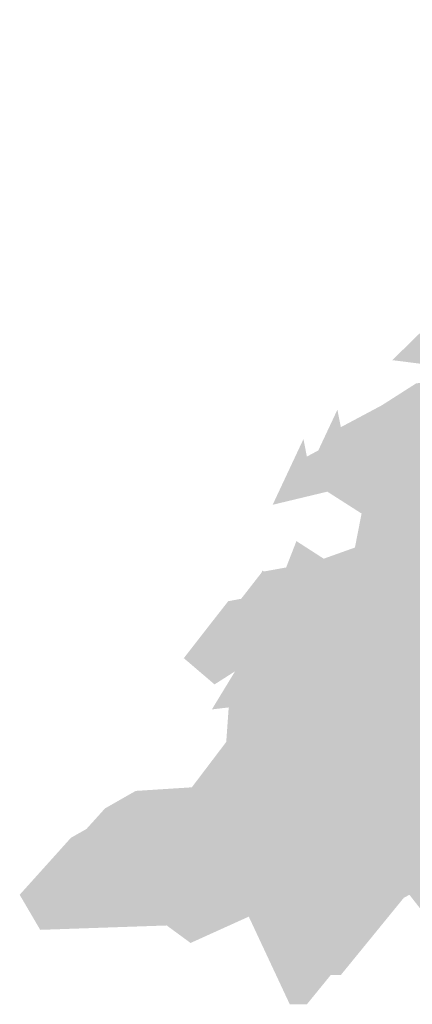
# Model space of a CAD drawing. Units: feet. Extents: x 2368 to 3224, y 836 to 1229.
# Tile 1 of 9: x 2390.53 to 2394.66, y 849.57 to 859.93. Entities that reach past the tile are written whole.
import ezdxf

# ---------------------------------------------------------------- set-up
doc = ezdxf.new("R2010")
doc.units = ezdxf.units.FT
doc.layers.add('L-PLNT', color=3, linetype='Continuous', lineweight=13)

msp = doc.modelspace()

# ---------------------------------------------------------------- hatches: boundary and pattern name
at = {"layer": 'L-PLNT'}
h = msp.add_hatch(color=256, dxfattribs=at)
h.dxf.hatch_style = 1
h.paths.add_polyline_path([(2401.097, 854.492), (2400.522, 855.091), (2399.803, 855.321), (2400.126, 855.828), (2399.839, 856.704), (2399.659, 856.704), (2399.3, 857.487), (2399.084, 857.441), (2398.832, 857.441), (2398.653, 857.809), (2398.76, 858.316), (2399.048, 858.316), (2398.509, 858.962), (2398.436, 859.473), (2398.149, 859.791), (2397.898, 859.514), (2397.754, 859.607), (2397.718, 859.837), (2397.538, 859.929), (2397.287, 859.699), (2396.999, 859.745), (2396.783, 859.33), (2396.783, 858.962), (2397.071, 858.823), (2396.855, 858.685), (2396.64, 858.869), (2396.029, 858.27), (2396.029, 858.132), (2395.777, 857.994), (2395.849, 857.856), (2396.029, 857.579), (2395.705, 857.349), (2395.382, 857.579), (2395.202, 857.533), (2395.13, 857.349), (2395.382, 857.303), (2395.418, 856.934), (2395.136, 856.98), (2394.806, 856.657), (2395.166, 856.611), (2395.022, 856.151), (2394.699, 856.104), (2394.339, 855.874), (2393.908, 855.644), (2393.872, 855.828), (2393.548, 855.137), (2394.124, 855.275), (2394.483, 855.045), (2394.375, 854.492), (2393.728, 854.261), (2393.441, 854.446), (2393.333, 854.169), (2393.081, 854.123), (2392.865, 853.846), (2392.614, 853.524), (2392.937, 853.247), (2393.153, 853.386), (2392.909, 852.985), (2393.086, 853.006), (2393.061, 852.643), (2392.47, 851.865), (2391.751, 851.819), (2391.428, 851.635), (2390.888, 851.035), (2391.104, 850.667), (2392.434, 850.713), (2392.686, 850.529), (2393.297, 850.805), (2393.728, 849.883), (2393.908, 849.883), (2394.735, 850.897), (2394.986, 851.035), (2395.166, 850.805), (2395.166, 850.483), (2395.453, 850.39), (2395.849, 850.39), (2395.993, 850.713), (2396.46, 850.943), (2396.927, 850.989), (2397.143, 851.174), (2397.179, 851.22), (2397.287, 851.45), (2397.43, 851.358), (2397.538, 850.989), (2397.79, 851.128), (2397.862, 851.035), (2397.934, 850.805), (2398.185, 851.22), (2398.437, 851.22), (2398.545, 851.035), (2398.437, 850.851), (2398.724, 850.943), (2398.832, 850.805), (2399.084, 850.989), (2399.336, 850.897), (2399.839, 850.39), (2400.054, 850.298), (2400.234, 850.114), (2401.744, 850.252), (2402.031, 849.976), (2402.247, 850.068), (2401.672, 850.805), (2401.636, 851.082), (2401.816, 851.358), (2401.492, 852.234), (2401.312, 852.234), (2400.953, 853.524), (2400.594, 853.57), (2400.809, 853.754)])
h = msp.add_hatch(color=256, dxfattribs=at)
h.dxf.hatch_style = 1
h.paths.add_polyline_path([(2400.74, 854.183), (2400.164, 854.782), (2399.446, 855.013), (2399.769, 855.519), (2399.482, 856.395), (2399.302, 856.395), (2398.942, 857.178), (2398.727, 857.132), (2398.475, 857.132), (2398.295, 857.501), (2398.403, 858.008), (2398.691, 858.008), (2398.152, 858.653), (2398.079, 859.164), (2397.792, 859.482), (2397.54, 859.206), (2397.397, 859.298), (2397.361, 859.529), (2397.181, 859.621), (2396.929, 859.39), (2396.642, 859.436), (2396.426, 859.022), (2396.426, 858.653), (2396.714, 858.515), (2396.498, 858.377), (2396.282, 858.561), (2395.671, 857.962), (2395.671, 857.824), (2395.42, 857.685), (2395.492, 857.547), (2395.671, 857.271), (2395.348, 857.04), (2395.024, 857.271), (2394.845, 857.224), (2394.773, 857.04), (2395.024, 856.994), (2395.06, 856.625), (2394.779, 856.672), (2394.449, 856.349), (2394.809, 856.303), (2394.665, 855.842), (2394.341, 855.796), (2393.982, 855.566), (2393.551, 855.335), (2393.515, 855.519), (2393.191, 854.828), (2393.766, 854.966), (2394.126, 854.736), (2394.018, 854.183), (2393.371, 853.953), (2393.083, 854.137), (2392.975, 853.861), (2392.724, 853.814), (2392.508, 853.538), (2392.257, 853.215), (2392.58, 852.939), (2392.796, 853.077), (2392.552, 852.676), (2392.729, 852.697), (2392.703, 852.334), (2392.113, 851.556), (2391.394, 851.51), (2391.07, 851.326), (2390.531, 850.727), (2390.747, 850.358), (2392.077, 850.404), (2392.328, 850.22), (2392.94, 850.497), (2393.371, 849.575), (2393.551, 849.575), (2394.377, 850.589), (2394.629, 850.727), (2394.809, 850.497), (2394.809, 850.174), (2395.096, 850.082), (2395.492, 850.082), (2395.635, 850.404), (2396.103, 850.635), (2396.57, 850.681), (2396.786, 850.865), (2396.822, 850.911), (2396.929, 851.142), (2397.073, 851.05), (2397.181, 850.681), (2397.433, 850.819), (2397.505, 850.727), (2397.576, 850.497), (2397.828, 850.911), (2398.08, 850.911), (2398.187, 850.727), (2398.08, 850.543), (2398.367, 850.635), (2398.475, 850.497), (2398.727, 850.681), (2398.978, 850.589), (2399.482, 850.082), (2399.697, 849.99), (2399.877, 849.805), (2401.387, 849.944), (2401.674, 849.667), (2401.89, 849.759), (2401.315, 850.497), (2401.279, 850.773), (2401.458, 851.05), (2401.135, 851.925), (2400.955, 851.925), (2400.596, 853.215), (2400.236, 853.261), (2400.452, 853.446)])

doc.saveas('drawing.dxf')
